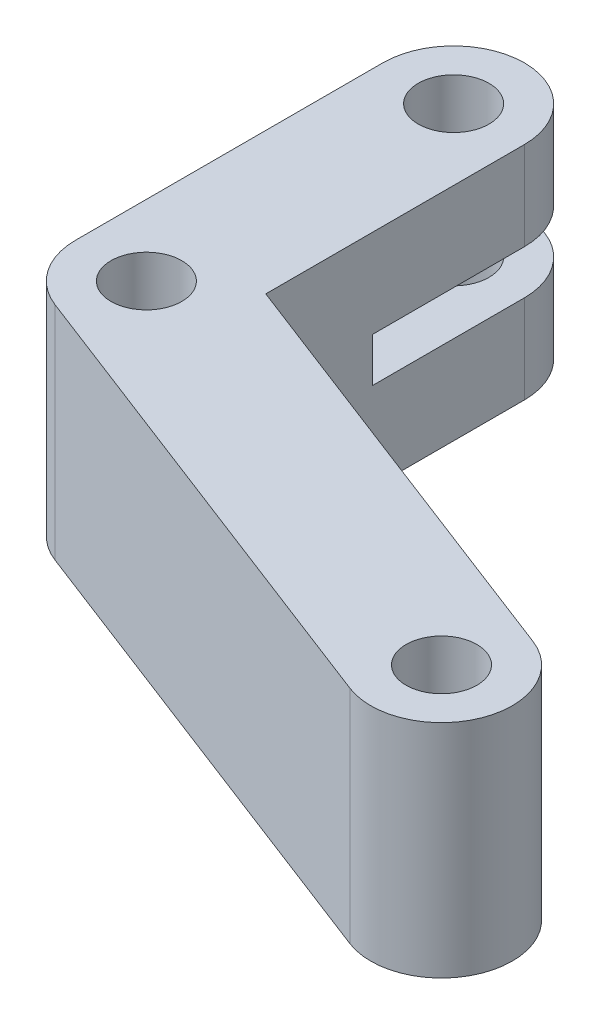
SolidWorks part; units mm, degrees
material "Plain Carbon Steel"
ref_plane "Front Plane" through (0, 0, 0) normal (0, 0, 1) x (1, 0, 0)
ref_plane "Top Plane" through (0, 0, 0) normal (0, 1, 0) x (1, 0, 0)
ref_plane "Right Plane" through (0, 0, 0) normal (1, 0, 0) x (0, 0, -1)
sketch "Bracket Profile Sketch" plane through (0, 0, 0) normal (0, 1, 0) x (1, 0, 0)
  line L0 (-593.2688, 0) -> (29070.1731, 0) construction
  line L1 (0, -593.2688) -> (0, 29070.1731) construction
  line L2 (0, 34.72) -> (0, 0) construction
  line L3 (8, 34.72) -> (8, 5.4917)
  line L4 (-8, 34.72) -> (-8, 0)
  line L5 (0, 0) -> (54.24, -20.89) construction
  line L6 (8, 5.4917) -> (57.1152, -13.4245)
  line L7 (-2.8752, -7.4655) -> (51.3648, -28.3555)
  arc A0 (8, 34.72) -> (-8, 34.72) centre (0, 34.72) ccw
  arc A1 (-8, 0) -> (-2.8752, -7.4655) centre (0, 0) ccw
  arc A3 (51.3648, -28.3555) -> (57.1152, -13.4245) centre (54.24, -20.89) ccw
  point P7 (0, 17.36)
  point P9 (-8, 17.36)
  point P12 (27.12, -10.445)
  dimension "D1" = 8
  dimension "D2" = 8
  dimension "D6" = 8
  dimension "D3" = 20.89
  dimension "D4" = 54.24
  dimension "D5" = 34.72
  dimension "D7" = 29.2283
  dimension "D8" = 16
  dimension "D9" = 16
  dimension "D10" = 49.1152
  dimension "D11" = 54.24
extrude "L Bracket Body" add sketch "Bracket Profile Sketch" along normal blind 25
sketch "Pivot Holes Sketch" plane through (0, 25, 0) normal (0, 1, 0) x (1, 0, 0)
  circle A0 centre (0, 34.72) radius 4
  circle A1 centre (54.24, -20.89) radius 4
  circle A2 centre (0, 0) radius 4
  dimension "D1" = 8
  dimension "D2" = 8
  dimension "D3" = 8
extrude "Pivot Holes 3xØ8" cut sketch "Pivot Holes Sketch" against normal blind 25
sketch "Clevis Slot Sketch" plane through (0, 0, 0) normal (1, 0, 0) x (0, 0, -1)
  line L0 (34.72, 0) -> (42.72, 0) construction
  line L1 (42.72, 15) -> (17.57, 15)
  line L2 (42.72, 15) -> (42.72, 10)
  line L3 (42.72, 10) -> (17.57, 10)
  line L4 (17.57, 15) -> (17.57, 10)
  line L5 (42.72, 0) -> (42.72, 25) construction
  point P4 (42.72, 12.5)
  dimension "D1" = 5
  dimension "D2" = 25.15
  dimension "D3" = 12.5
extrude "Clevis Slot 5mm" cut sketch "Clevis Slot Sketch" against normal mid plane 25
